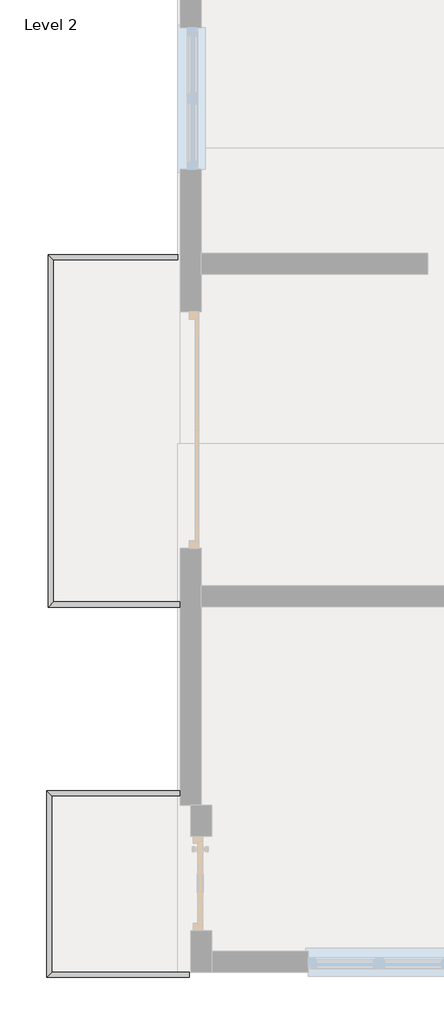
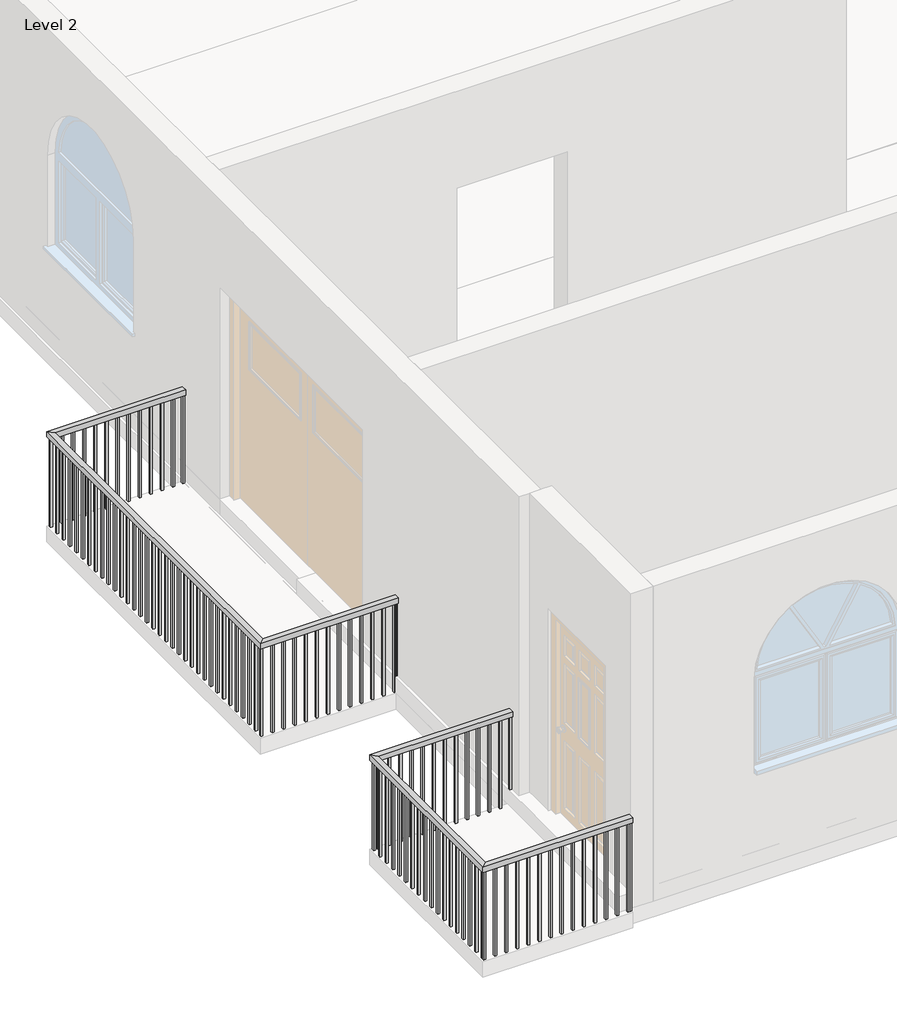
# One storey, part 3 of 7: 2 railings.
"""IFC4 building model written with IfcOpenShell, lengths in millimetres."""

from ifc_helpers import new_model, si_unit, frame, origin, place, context, project, spatial, polyline, outline, extrude, faceted_brep, element, save

model = new_model("IFC4")

# Units and contexts
model_context = context("Model", 3, world=origin())
ifc_project = project(units=[si_unit("LENGTHUNIT", "METRE", prefix="MILLI")], contexts=[model_context])

# Site, building, storey
site = spatial("IfcSite", under=ifc_project)
building = spatial("IfcBuilding", under=site)
storey = spatial("IfcBuildingStorey", under=building, Name="Level 2", Elevation=3048.0)

# Railings
placement = place(None, origin())
element("IfcRailing", 1, ObjectType="Handrail - Rectangular", at=placement, inside=storey, context=model_context, shape_type="SolidModel", body=[
    faceted_brep([(-6354.2109037, -3767.6037749, 3962.4), (-6354.2109037, -3767.6037749, 3911.6), (-6354.2109037, -3716.8037749, 3911.6), (-6354.2109037, -3716.8037749, 3962.4), (-7548.0109037, -3767.6037749, 3962.4), (-7548.0109037, -3767.6037749, 3911.6), (-7598.8109037, -3716.8037749, 3911.6), (-7598.8109037, -3716.8037749, 3962.4), (-7548.0109037, -7054.4894702, 3962.4), (-7548.0109037, -7054.4894702, 3911.6), (-7598.8109037, -7105.2894702, 3911.6), (-7598.8109037, -7105.2894702, 3962.4), (-6330.8013636, -7054.4894702, 3962.4), (-6330.8013636, -7105.2894702, 3962.4), (-6330.8013636, -7105.2894702, 3911.6), (-6330.8013636, -7054.4894702, 3911.6)], [[[0, 1, 2, 3]], [[1, 0, 4, 5]], [[2, 1, 5, 6]], [[3, 2, 6, 7]], [[0, 3, 7, 4]], [[5, 4, 8, 9]], [[6, 5, 9, 10]], [[7, 6, 10, 11]], [[4, 7, 11, 8]], [[12, 13, 14, 15]], [[9, 8, 12, 15]], [[10, 9, 15, 14]], [[11, 10, 14, 13]], [[8, 11, 13, 12]]]),
    extrude(outline(polyline([(-6363.7359037, -7089.4144702), (-6363.7359037, -7070.3644702), (-6344.6859037, -7070.3644702), (-6344.6859037, -7089.4144702), (-6363.7359037, -7089.4144702)])), frame((0.0, 0.0, 3048.0), z_axis=(0.0, 0.0, 1.0), x_axis=(1.0, 0.0, 0.0)), (0.0, 0.0, 1.0), 863.6),
    extrude(outline(polyline([(-6465.3359037, -7089.4144702), (-6465.3359037, -7070.3644702), (-6446.2859037, -7070.3644702), (-6446.2859037, -7089.4144702), (-6465.3359037, -7089.4144702)])), frame((0.0, 0.0, 3048.0), z_axis=(0.0, 0.0, 1.0), x_axis=(1.0, 0.0, 0.0)), (0.0, 0.0, 1.0), 863.6),
    extrude(outline(polyline([(-6566.9359037, -7089.4144702), (-6566.9359037, -7070.3644702), (-6547.8859037, -7070.3644702), (-6547.8859037, -7089.4144702), (-6566.9359037, -7089.4144702)])), frame((0.0, 0.0, 3048.0), z_axis=(0.0, 0.0, 1.0), x_axis=(1.0, 0.0, 0.0)), (0.0, 0.0, 1.0), 863.6),
    extrude(outline(polyline([(-6668.5359037, -7089.4144702), (-6668.5359037, -7070.3644702), (-6649.4859037, -7070.3644702), (-6649.4859037, -7089.4144702), (-6668.5359037, -7089.4144702)])), frame((0.0, 0.0, 3048.0), z_axis=(0.0, 0.0, 1.0), x_axis=(1.0, 0.0, 0.0)), (0.0, 0.0, 1.0), 863.6),
    extrude(outline(polyline([(-6770.1359037, -7089.4144702), (-6770.1359037, -7070.3644702), (-6751.0859037, -7070.3644702), (-6751.0859037, -7089.4144702), (-6770.1359037, -7089.4144702)])), frame((0.0, 0.0, 3048.0), z_axis=(0.0, 0.0, 1.0), x_axis=(1.0, 0.0, 0.0)), (0.0, 0.0, 1.0), 863.6),
    extrude(outline(polyline([(-6871.7359037, -7089.4144702), (-6871.7359037, -7070.3644702), (-6852.6859037, -7070.3644702), (-6852.6859037, -7089.4144702), (-6871.7359037, -7089.4144702)])), frame((0.0, 0.0, 3048.0), z_axis=(0.0, 0.0, 1.0), x_axis=(1.0, 0.0, 0.0)), (0.0, 0.0, 1.0), 863.6),
    extrude(outline(polyline([(-6973.3359037, -7089.4144702), (-6973.3359037, -7070.3644702), (-6954.2859037, -7070.3644702), (-6954.2859037, -7089.4144702), (-6973.3359037, -7089.4144702)])), frame((0.0, 0.0, 3048.0), z_axis=(0.0, 0.0, 1.0), x_axis=(1.0, 0.0, 0.0)), (0.0, 0.0, 1.0), 863.6),
    extrude(outline(polyline([(-7074.9359037, -7089.4144702), (-7074.9359037, -7070.3644702), (-7055.8859037, -7070.3644702), (-7055.8859037, -7089.4144702), (-7074.9359037, -7089.4144702)])), frame((0.0, 0.0, 3048.0), z_axis=(0.0, 0.0, 1.0), x_axis=(1.0, 0.0, 0.0)), (0.0, 0.0, 1.0), 863.6),
    extrude(outline(polyline([(-7176.5359037, -7089.4144702), (-7176.5359037, -7070.3644702), (-7157.4859037, -7070.3644702), (-7157.4859037, -7089.4144702), (-7176.5359037, -7089.4144702)])), frame((0.0, 0.0, 3048.0), z_axis=(0.0, 0.0, 1.0), x_axis=(1.0, 0.0, 0.0)), (0.0, 0.0, 1.0), 863.6),
    extrude(outline(polyline([(-7278.1359037, -7089.4144702), (-7278.1359037, -7070.3644702), (-7259.0859037, -7070.3644702), (-7259.0859037, -7089.4144702), (-7278.1359037, -7089.4144702)])), frame((0.0, 0.0, 3048.0), z_axis=(0.0, 0.0, 1.0), x_axis=(1.0, 0.0, 0.0)), (0.0, 0.0, 1.0), 863.6),
    extrude(outline(polyline([(-7379.7359037, -7089.4144702), (-7379.7359037, -7070.3644702), (-7360.6859037, -7070.3644702), (-7360.6859037, -7089.4144702), (-7379.7359037, -7089.4144702)])), frame((0.0, 0.0, 3048.0), z_axis=(0.0, 0.0, 1.0), x_axis=(1.0, 0.0, 0.0)), (0.0, 0.0, 1.0), 863.6),
    extrude(outline(polyline([(-7481.3359037, -7089.4144702), (-7481.3359037, -7070.3644702), (-7462.2859037, -7070.3644702), (-7462.2859037, -7089.4144702), (-7481.3359037, -7089.4144702)])), frame((0.0, 0.0, 3048.0), z_axis=(0.0, 0.0, 1.0), x_axis=(1.0, 0.0, 0.0)), (0.0, 0.0, 1.0), 863.6),
    extrude(outline(polyline([(-7582.9359037, -6983.8787749), (-7563.8859037, -6983.8787749), (-7563.8859037, -7002.9287749), (-7582.9359037, -7002.9287749), (-7582.9359037, -6983.8787749)])), frame((0.0, 0.0, 3048.0), z_axis=(0.0, 0.0, 1.0), x_axis=(1.0, 0.0, 0.0)), (0.0, 0.0, 1.0), 863.6),
    extrude(outline(polyline([(-7582.9359037, -6882.2787749), (-7563.8859037, -6882.2787749), (-7563.8859037, -6901.3287749), (-7582.9359037, -6901.3287749), (-7582.9359037, -6882.2787749)])), frame((0.0, 0.0, 3048.0), z_axis=(0.0, 0.0, 1.0), x_axis=(1.0, 0.0, 0.0)), (0.0, 0.0, 1.0), 863.6),
    extrude(outline(polyline([(-7582.9359037, -6780.6787749), (-7563.8859037, -6780.6787749), (-7563.8859037, -6799.7287749), (-7582.9359037, -6799.7287749), (-7582.9359037, -6780.6787749)])), frame((0.0, 0.0, 3048.0), z_axis=(0.0, 0.0, 1.0), x_axis=(1.0, 0.0, 0.0)), (0.0, 0.0, 1.0), 863.6),
    extrude(outline(polyline([(-7582.9359037, -6679.0787749), (-7563.8859037, -6679.0787749), (-7563.8859037, -6698.1287749), (-7582.9359037, -6698.1287749), (-7582.9359037, -6679.0787749)])), frame((0.0, 0.0, 3048.0), z_axis=(0.0, 0.0, 1.0), x_axis=(1.0, 0.0, 0.0)), (0.0, 0.0, 1.0), 863.6),
    extrude(outline(polyline([(-7582.9359037, -6577.4787749), (-7563.8859037, -6577.4787749), (-7563.8859037, -6596.5287749), (-7582.9359037, -6596.5287749), (-7582.9359037, -6577.4787749)])), frame((0.0, 0.0, 3048.0), z_axis=(0.0, 0.0, 1.0), x_axis=(1.0, 0.0, 0.0)), (0.0, 0.0, 1.0), 863.6),
    extrude(outline(polyline([(-7582.9359037, -6475.8787749), (-7563.8859037, -6475.8787749), (-7563.8859037, -6494.9287749), (-7582.9359037, -6494.9287749), (-7582.9359037, -6475.8787749)])), frame((0.0, 0.0, 3048.0), z_axis=(0.0, 0.0, 1.0), x_axis=(1.0, 0.0, 0.0)), (0.0, 0.0, 1.0), 863.6),
    extrude(outline(polyline([(-7582.9359037, -6374.2787749), (-7563.8859037, -6374.2787749), (-7563.8859037, -6393.3287749), (-7582.9359037, -6393.3287749), (-7582.9359037, -6374.2787749)])), frame((0.0, 0.0, 3048.0), z_axis=(0.0, 0.0, 1.0), x_axis=(1.0, 0.0, 0.0)), (0.0, 0.0, 1.0), 863.6),
    extrude(outline(polyline([(-7582.9359037, -6272.6787749), (-7563.8859037, -6272.6787749), (-7563.8859037, -6291.7287749), (-7582.9359037, -6291.7287749), (-7582.9359037, -6272.6787749)])), frame((0.0, 0.0, 3048.0), z_axis=(0.0, 0.0, 1.0), x_axis=(1.0, 0.0, 0.0)), (0.0, 0.0, 1.0), 863.6),
    extrude(outline(polyline([(-7582.9359037, -6171.0787749), (-7563.8859037, -6171.0787749), (-7563.8859037, -6190.1287749), (-7582.9359037, -6190.1287749), (-7582.9359037, -6171.0787749)])), frame((0.0, 0.0, 3048.0), z_axis=(0.0, 0.0, 1.0), x_axis=(1.0, 0.0, 0.0)), (0.0, 0.0, 1.0), 863.6),
    extrude(outline(polyline([(-7582.9359037, -6069.4787749), (-7563.8859037, -6069.4787749), (-7563.8859037, -6088.5287749), (-7582.9359037, -6088.5287749), (-7582.9359037, -6069.4787749)])), frame((0.0, 0.0, 3048.0), z_axis=(0.0, 0.0, 1.0), x_axis=(1.0, 0.0, 0.0)), (0.0, 0.0, 1.0), 863.6),
    extrude(outline(polyline([(-7582.9359037, -5967.8787749), (-7563.8859037, -5967.8787749), (-7563.8859037, -5986.9287749), (-7582.9359037, -5986.9287749), (-7582.9359037, -5967.8787749)])), frame((0.0, 0.0, 3048.0), z_axis=(0.0, 0.0, 1.0), x_axis=(1.0, 0.0, 0.0)), (0.0, 0.0, 1.0), 863.6),
    extrude(outline(polyline([(-7582.9359037, -5866.2787749), (-7563.8859037, -5866.2787749), (-7563.8859037, -5885.3287749), (-7582.9359037, -5885.3287749), (-7582.9359037, -5866.2787749)])), frame((0.0, 0.0, 3048.0), z_axis=(0.0, 0.0, 1.0), x_axis=(1.0, 0.0, 0.0)), (0.0, 0.0, 1.0), 863.6),
    extrude(outline(polyline([(-7582.9359037, -5764.6787749), (-7563.8859037, -5764.6787749), (-7563.8859037, -5783.7287749), (-7582.9359037, -5783.7287749), (-7582.9359037, -5764.6787749)])), frame((0.0, 0.0, 3048.0), z_axis=(0.0, 0.0, 1.0), x_axis=(1.0, 0.0, 0.0)), (0.0, 0.0, 1.0), 863.6),
    extrude(outline(polyline([(-7582.9359037, -5663.0787749), (-7563.8859037, -5663.0787749), (-7563.8859037, -5682.1287749), (-7582.9359037, -5682.1287749), (-7582.9359037, -5663.0787749)])), frame((0.0, 0.0, 3048.0), z_axis=(0.0, 0.0, 1.0), x_axis=(1.0, 0.0, 0.0)), (0.0, 0.0, 1.0), 863.6),
    extrude(outline(polyline([(-7582.9359037, -5561.4787749), (-7563.8859037, -5561.4787749), (-7563.8859037, -5580.5287749), (-7582.9359037, -5580.5287749), (-7582.9359037, -5561.4787749)])), frame((0.0, 0.0, 3048.0), z_axis=(0.0, 0.0, 1.0), x_axis=(1.0, 0.0, 0.0)), (0.0, 0.0, 1.0), 863.6),
    extrude(outline(polyline([(-7582.9359037, -5459.8787749), (-7563.8859037, -5459.8787749), (-7563.8859037, -5478.9287749), (-7582.9359037, -5478.9287749), (-7582.9359037, -5459.8787749)])), frame((0.0, 0.0, 3048.0), z_axis=(0.0, 0.0, 1.0), x_axis=(1.0, 0.0, 0.0)), (0.0, 0.0, 1.0), 863.6),
    extrude(outline(polyline([(-7582.9359037, -5358.2787749), (-7563.8859037, -5358.2787749), (-7563.8859037, -5377.3287749), (-7582.9359037, -5377.3287749), (-7582.9359037, -5358.2787749)])), frame((0.0, 0.0, 3048.0), z_axis=(0.0, 0.0, 1.0), x_axis=(1.0, 0.0, 0.0)), (0.0, 0.0, 1.0), 863.6),
    extrude(outline(polyline([(-7582.9359037, -5256.6787749), (-7563.8859037, -5256.6787749), (-7563.8859037, -5275.7287749), (-7582.9359037, -5275.7287749), (-7582.9359037, -5256.6787749)])), frame((0.0, 0.0, 3048.0), z_axis=(0.0, 0.0, 1.0), x_axis=(1.0, 0.0, 0.0)), (0.0, 0.0, 1.0), 863.6),
    extrude(outline(polyline([(-7582.9359037, -5155.0787749), (-7563.8859037, -5155.0787749), (-7563.8859037, -5174.1287749), (-7582.9359037, -5174.1287749), (-7582.9359037, -5155.0787749)])), frame((0.0, 0.0, 3048.0), z_axis=(0.0, 0.0, 1.0), x_axis=(1.0, 0.0, 0.0)), (0.0, 0.0, 1.0), 863.6),
    extrude(outline(polyline([(-7582.9359037, -5053.4787749), (-7563.8859037, -5053.4787749), (-7563.8859037, -5072.5287749), (-7582.9359037, -5072.5287749), (-7582.9359037, -5053.4787749)])), frame((0.0, 0.0, 3048.0), z_axis=(0.0, 0.0, 1.0), x_axis=(1.0, 0.0, 0.0)), (0.0, 0.0, 1.0), 863.6),
    extrude(outline(polyline([(-7582.9359037, -4951.8787749), (-7563.8859037, -4951.8787749), (-7563.8859037, -4970.9287749), (-7582.9359037, -4970.9287749), (-7582.9359037, -4951.8787749)])), frame((0.0, 0.0, 3048.0), z_axis=(0.0, 0.0, 1.0), x_axis=(1.0, 0.0, 0.0)), (0.0, 0.0, 1.0), 863.6),
    extrude(outline(polyline([(-7582.9359037, -4850.2787749), (-7563.8859037, -4850.2787749), (-7563.8859037, -4869.3287749), (-7582.9359037, -4869.3287749), (-7582.9359037, -4850.2787749)])), frame((0.0, 0.0, 3048.0), z_axis=(0.0, 0.0, 1.0), x_axis=(1.0, 0.0, 0.0)), (0.0, 0.0, 1.0), 863.6),
    extrude(outline(polyline([(-7582.9359037, -4748.6787749), (-7563.8859037, -4748.6787749), (-7563.8859037, -4767.7287749), (-7582.9359037, -4767.7287749), (-7582.9359037, -4748.6787749)])), frame((0.0, 0.0, 3048.0), z_axis=(0.0, 0.0, 1.0), x_axis=(1.0, 0.0, 0.0)), (0.0, 0.0, 1.0), 863.6),
    extrude(outline(polyline([(-7582.9359037, -4647.0787749), (-7563.8859037, -4647.0787749), (-7563.8859037, -4666.1287749), (-7582.9359037, -4666.1287749), (-7582.9359037, -4647.0787749)])), frame((0.0, 0.0, 3048.0), z_axis=(0.0, 0.0, 1.0), x_axis=(1.0, 0.0, 0.0)), (0.0, 0.0, 1.0), 863.6),
    extrude(outline(polyline([(-7582.9359037, -4545.4787749), (-7563.8859037, -4545.4787749), (-7563.8859037, -4564.5287749), (-7582.9359037, -4564.5287749), (-7582.9359037, -4545.4787749)])), frame((0.0, 0.0, 3048.0), z_axis=(0.0, 0.0, 1.0), x_axis=(1.0, 0.0, 0.0)), (0.0, 0.0, 1.0), 863.6),
    extrude(outline(polyline([(-7582.9359037, -4443.8787749), (-7563.8859037, -4443.8787749), (-7563.8859037, -4462.9287749), (-7582.9359037, -4462.9287749), (-7582.9359037, -4443.8787749)])), frame((0.0, 0.0, 3048.0), z_axis=(0.0, 0.0, 1.0), x_axis=(1.0, 0.0, 0.0)), (0.0, 0.0, 1.0), 863.6),
    extrude(outline(polyline([(-7582.9359037, -4342.2787749), (-7563.8859037, -4342.2787749), (-7563.8859037, -4361.3287749), (-7582.9359037, -4361.3287749), (-7582.9359037, -4342.2787749)])), frame((0.0, 0.0, 3048.0), z_axis=(0.0, 0.0, 1.0), x_axis=(1.0, 0.0, 0.0)), (0.0, 0.0, 1.0), 863.6),
    extrude(outline(polyline([(-7582.9359037, -4240.6787749), (-7563.8859037, -4240.6787749), (-7563.8859037, -4259.7287749), (-7582.9359037, -4259.7287749), (-7582.9359037, -4240.6787749)])), frame((0.0, 0.0, 3048.0), z_axis=(0.0, 0.0, 1.0), x_axis=(1.0, 0.0, 0.0)), (0.0, 0.0, 1.0), 863.6),
    extrude(outline(polyline([(-7582.9359037, -4139.0787749), (-7563.8859037, -4139.0787749), (-7563.8859037, -4158.1287749), (-7582.9359037, -4158.1287749), (-7582.9359037, -4139.0787749)])), frame((0.0, 0.0, 3048.0), z_axis=(0.0, 0.0, 1.0), x_axis=(1.0, 0.0, 0.0)), (0.0, 0.0, 1.0), 863.6),
    extrude(outline(polyline([(-7582.9359037, -4037.4787749), (-7563.8859037, -4037.4787749), (-7563.8859037, -4056.5287749), (-7582.9359037, -4056.5287749), (-7582.9359037, -4037.4787749)])), frame((0.0, 0.0, 3048.0), z_axis=(0.0, 0.0, 1.0), x_axis=(1.0, 0.0, 0.0)), (0.0, 0.0, 1.0), 863.6),
    extrude(outline(polyline([(-7582.9359037, -3935.8787749), (-7563.8859037, -3935.8787749), (-7563.8859037, -3954.9287749), (-7582.9359037, -3954.9287749), (-7582.9359037, -3935.8787749)])), frame((0.0, 0.0, 3048.0), z_axis=(0.0, 0.0, 1.0), x_axis=(1.0, 0.0, 0.0)), (0.0, 0.0, 1.0), 863.6),
    extrude(outline(polyline([(-7582.9359037, -3834.2787749), (-7563.8859037, -3834.2787749), (-7563.8859037, -3853.3287749), (-7582.9359037, -3853.3287749), (-7582.9359037, -3834.2787749)])), frame((0.0, 0.0, 3048.0), z_axis=(0.0, 0.0, 1.0), x_axis=(1.0, 0.0, 0.0)), (0.0, 0.0, 1.0), 863.6),
    extrude(outline(polyline([(-7462.2859037, -3732.6787749), (-7462.2859037, -3751.7287749), (-7481.3359037, -3751.7287749), (-7481.3359037, -3732.6787749), (-7462.2859037, -3732.6787749)])), frame((0.0, 0.0, 3048.0), z_axis=(0.0, 0.0, 1.0), x_axis=(1.0, 0.0, 0.0)), (0.0, 0.0, 1.0), 863.6),
    extrude(outline(polyline([(-7360.6859037, -3732.6787749), (-7360.6859037, -3751.7287749), (-7379.7359037, -3751.7287749), (-7379.7359037, -3732.6787749), (-7360.6859037, -3732.6787749)])), frame((0.0, 0.0, 3048.0), z_axis=(0.0, 0.0, 1.0), x_axis=(1.0, 0.0, 0.0)), (0.0, 0.0, 1.0), 863.6),
    extrude(outline(polyline([(-7259.0859037, -3732.6787749), (-7259.0859037, -3751.7287749), (-7278.1359037, -3751.7287749), (-7278.1359037, -3732.6787749), (-7259.0859037, -3732.6787749)])), frame((0.0, 0.0, 3048.0), z_axis=(0.0, 0.0, 1.0), x_axis=(1.0, 0.0, 0.0)), (0.0, 0.0, 1.0), 863.6),
    extrude(outline(polyline([(-7157.4859037, -3732.6787749), (-7157.4859037, -3751.7287749), (-7176.5359037, -3751.7287749), (-7176.5359037, -3732.6787749), (-7157.4859037, -3732.6787749)])), frame((0.0, 0.0, 3048.0), z_axis=(0.0, 0.0, 1.0), x_axis=(1.0, 0.0, 0.0)), (0.0, 0.0, 1.0), 863.6),
    extrude(outline(polyline([(-7055.8859037, -3732.6787749), (-7055.8859037, -3751.7287749), (-7074.9359037, -3751.7287749), (-7074.9359037, -3732.6787749), (-7055.8859037, -3732.6787749)])), frame((0.0, 0.0, 3048.0), z_axis=(0.0, 0.0, 1.0), x_axis=(1.0, 0.0, 0.0)), (0.0, 0.0, 1.0), 863.6),
    extrude(outline(polyline([(-6954.2859037, -3732.6787749), (-6954.2859037, -3751.7287749), (-6973.3359037, -3751.7287749), (-6973.3359037, -3732.6787749), (-6954.2859037, -3732.6787749)])), frame((0.0, 0.0, 3048.0), z_axis=(0.0, 0.0, 1.0), x_axis=(1.0, 0.0, 0.0)), (0.0, 0.0, 1.0), 863.6),
    extrude(outline(polyline([(-6852.6859037, -3732.6787749), (-6852.6859037, -3751.7287749), (-6871.7359037, -3751.7287749), (-6871.7359037, -3732.6787749), (-6852.6859037, -3732.6787749)])), frame((0.0, 0.0, 3048.0), z_axis=(0.0, 0.0, 1.0), x_axis=(1.0, 0.0, 0.0)), (0.0, 0.0, 1.0), 863.6),
    extrude(outline(polyline([(-6751.0859037, -3732.6787749), (-6751.0859037, -3751.7287749), (-6770.1359037, -3751.7287749), (-6770.1359037, -3732.6787749), (-6751.0859037, -3732.6787749)])), frame((0.0, 0.0, 3048.0), z_axis=(0.0, 0.0, 1.0), x_axis=(1.0, 0.0, 0.0)), (0.0, 0.0, 1.0), 863.6),
    extrude(outline(polyline([(-6649.4859037, -3732.6787749), (-6649.4859037, -3751.7287749), (-6668.5359037, -3751.7287749), (-6668.5359037, -3732.6787749), (-6649.4859037, -3732.6787749)])), frame((0.0, 0.0, 3048.0), z_axis=(0.0, 0.0, 1.0), x_axis=(1.0, 0.0, 0.0)), (0.0, 0.0, 1.0), 863.6),
    extrude(outline(polyline([(-6547.8859037, -3732.6787749), (-6547.8859037, -3751.7287749), (-6566.9359037, -3751.7287749), (-6566.9359037, -3732.6787749), (-6547.8859037, -3732.6787749)])), frame((0.0, 0.0, 3048.0), z_axis=(0.0, 0.0, 1.0), x_axis=(1.0, 0.0, 0.0)), (0.0, 0.0, 1.0), 863.6),
    extrude(outline(polyline([(-6446.2859037, -3732.6787749), (-6446.2859037, -3751.7287749), (-6465.3359037, -3751.7287749), (-6465.3359037, -3732.6787749), (-6446.2859037, -3732.6787749)])), frame((0.0, 0.0, 3048.0), z_axis=(0.0, 0.0, 1.0), x_axis=(1.0, 0.0, 0.0)), (0.0, 0.0, 1.0), 863.6),
    extrude(outline(polyline([(-7582.9359037, -7070.3644702), (-7563.8859037, -7070.3644702), (-7563.8859037, -7089.4144702), (-7582.9359037, -7089.4144702), (-7582.9359037, -7070.3644702)])), frame((0.0, 0.0, 3048.0), z_axis=(0.0, 0.0, 1.0), x_axis=(1.0, 0.0, 0.0)), (0.0, 0.0, 1.0), 863.6),
    extrude(outline(polyline([(-7563.8859037, -3732.6787749), (-7563.8859037, -3751.7287749), (-7582.9359037, -3751.7287749), (-7582.9359037, -3732.6787749), (-7563.8859037, -3732.6787749)])), frame((0.0, 0.0, 3048.0), z_axis=(0.0, 0.0, 1.0), x_axis=(1.0, 0.0, 0.0)), (0.0, 0.0, 1.0), 863.6),
    extrude(outline(polyline([(-6349.8513636, -7089.4144702), (-6349.8513636, -7070.3644702), (-6330.8013636, -7070.3644702), (-6330.8013636, -7089.4144702), (-6349.8513636, -7089.4144702)])), frame((0.0, 0.0, 3048.0), z_axis=(0.0, 0.0, 1.0), x_axis=(1.0, 0.0, 0.0)), (0.0, 0.0, 1.0), 863.6),
    extrude(outline(polyline([(-6354.2109037, -3732.6787749), (-6354.2109037, -3751.7287749), (-6373.2609037, -3751.7287749), (-6373.2609037, -3732.6787749), (-6354.2109037, -3732.6787749)])), frame((0.0, 0.0, 3048.0), z_axis=(0.0, 0.0, 1.0), x_axis=(1.0, 0.0, 0.0)), (0.0, 0.0, 1.0), 863.6),
])
element("IfcRailing", 2, ObjectType="Handrail - Rectangular", at=placement, inside=storey, context=model_context, shape_type="SolidModel", body=[
    faceted_brep([(-6330.8013636, -8918.8845215, 3962.4), (-6330.8013636, -8918.8845215, 3911.6), (-6330.8013636, -8868.0845215, 3911.6), (-6330.8013636, -8868.0845215, 3962.4), (-7563.8859037, -8918.8845215, 3962.4), (-7563.8859037, -8918.8845215, 3911.6), (-7614.6859037, -8868.0845215, 3911.6), (-7614.6859037, -8868.0845215, 3962.4), (-7563.8859037, -10612.9037749, 3962.4), (-7563.8859037, -10612.9037749, 3911.6), (-7614.6859037, -10663.7037749, 3911.6), (-7614.6859037, -10663.7037749, 3962.4), (-6243.0859037, -10612.9037749, 3962.4), (-6243.0859037, -10663.7037749, 3962.4), (-6243.0859037, -10663.7037749, 3911.6), (-6243.0859037, -10612.9037749, 3911.6)], [[[0, 1, 2, 3]], [[1, 0, 4, 5]], [[2, 1, 5, 6]], [[3, 2, 6, 7]], [[0, 3, 7, 4]], [[5, 4, 8, 9]], [[6, 5, 9, 10]], [[7, 6, 10, 11]], [[4, 7, 11, 8]], [[12, 13, 14, 15]], [[9, 8, 12, 15]], [[10, 9, 15, 14]], [[11, 10, 14, 13]], [[8, 11, 13, 12]]]),
    extrude(outline(polyline([(-6278.0109037, -10647.8287749), (-6278.0109037, -10628.7787749), (-6258.9609037, -10628.7787749), (-6258.9609037, -10647.8287749), (-6278.0109037, -10647.8287749)])), frame((0.0, 0.0, 3048.0), z_axis=(0.0, 0.0, 1.0), x_axis=(1.0, 0.0, 0.0)), (0.0, 0.0, 1.0), 863.6),
    extrude(outline(polyline([(-6379.6109037, -10647.8287749), (-6379.6109037, -10628.7787749), (-6360.5609037, -10628.7787749), (-6360.5609037, -10647.8287749), (-6379.6109037, -10647.8287749)])), frame((0.0, 0.0, 3048.0), z_axis=(0.0, 0.0, 1.0), x_axis=(1.0, 0.0, 0.0)), (0.0, 0.0, 1.0), 863.6),
    extrude(outline(polyline([(-6481.2109037, -10647.8287749), (-6481.2109037, -10628.7787749), (-6462.1609037, -10628.7787749), (-6462.1609037, -10647.8287749), (-6481.2109037, -10647.8287749)])), frame((0.0, 0.0, 3048.0), z_axis=(0.0, 0.0, 1.0), x_axis=(1.0, 0.0, 0.0)), (0.0, 0.0, 1.0), 863.6),
    extrude(outline(polyline([(-6582.8109037, -10647.8287749), (-6582.8109037, -10628.7787749), (-6563.7609037, -10628.7787749), (-6563.7609037, -10647.8287749), (-6582.8109037, -10647.8287749)])), frame((0.0, 0.0, 3048.0), z_axis=(0.0, 0.0, 1.0), x_axis=(1.0, 0.0, 0.0)), (0.0, 0.0, 1.0), 863.6),
    extrude(outline(polyline([(-6684.4109037, -10647.8287749), (-6684.4109037, -10628.7787749), (-6665.3609037, -10628.7787749), (-6665.3609037, -10647.8287749), (-6684.4109037, -10647.8287749)])), frame((0.0, 0.0, 3048.0), z_axis=(0.0, 0.0, 1.0), x_axis=(1.0, 0.0, 0.0)), (0.0, 0.0, 1.0), 863.6),
    extrude(outline(polyline([(-6786.0109037, -10647.8287749), (-6786.0109037, -10628.7787749), (-6766.9609037, -10628.7787749), (-6766.9609037, -10647.8287749), (-6786.0109037, -10647.8287749)])), frame((0.0, 0.0, 3048.0), z_axis=(0.0, 0.0, 1.0), x_axis=(1.0, 0.0, 0.0)), (0.0, 0.0, 1.0), 863.6),
    extrude(outline(polyline([(-6887.6109037, -10647.8287749), (-6887.6109037, -10628.7787749), (-6868.5609037, -10628.7787749), (-6868.5609037, -10647.8287749), (-6887.6109037, -10647.8287749)])), frame((0.0, 0.0, 3048.0), z_axis=(0.0, 0.0, 1.0), x_axis=(1.0, 0.0, 0.0)), (0.0, 0.0, 1.0), 863.6),
    extrude(outline(polyline([(-6989.2109037, -10647.8287749), (-6989.2109037, -10628.7787749), (-6970.1609037, -10628.7787749), (-6970.1609037, -10647.8287749), (-6989.2109037, -10647.8287749)])), frame((0.0, 0.0, 3048.0), z_axis=(0.0, 0.0, 1.0), x_axis=(1.0, 0.0, 0.0)), (0.0, 0.0, 1.0), 863.6),
    extrude(outline(polyline([(-7090.8109037, -10647.8287749), (-7090.8109037, -10628.7787749), (-7071.7609037, -10628.7787749), (-7071.7609037, -10647.8287749), (-7090.8109037, -10647.8287749)])), frame((0.0, 0.0, 3048.0), z_axis=(0.0, 0.0, 1.0), x_axis=(1.0, 0.0, 0.0)), (0.0, 0.0, 1.0), 863.6),
    extrude(outline(polyline([(-7192.4109037, -10647.8287749), (-7192.4109037, -10628.7787749), (-7173.3609037, -10628.7787749), (-7173.3609037, -10647.8287749), (-7192.4109037, -10647.8287749)])), frame((0.0, 0.0, 3048.0), z_axis=(0.0, 0.0, 1.0), x_axis=(1.0, 0.0, 0.0)), (0.0, 0.0, 1.0), 863.6),
    extrude(outline(polyline([(-7294.0109037, -10647.8287749), (-7294.0109037, -10628.7787749), (-7274.9609037, -10628.7787749), (-7274.9609037, -10647.8287749), (-7294.0109037, -10647.8287749)])), frame((0.0, 0.0, 3048.0), z_axis=(0.0, 0.0, 1.0), x_axis=(1.0, 0.0, 0.0)), (0.0, 0.0, 1.0), 863.6),
    extrude(outline(polyline([(-7395.6109037, -10647.8287749), (-7395.6109037, -10628.7787749), (-7376.5609037, -10628.7787749), (-7376.5609037, -10647.8287749), (-7395.6109037, -10647.8287749)])), frame((0.0, 0.0, 3048.0), z_axis=(0.0, 0.0, 1.0), x_axis=(1.0, 0.0, 0.0)), (0.0, 0.0, 1.0), 863.6),
    extrude(outline(polyline([(-7497.2109037, -10647.8287749), (-7497.2109037, -10628.7787749), (-7478.1609037, -10628.7787749), (-7478.1609037, -10647.8287749), (-7497.2109037, -10647.8287749)])), frame((0.0, 0.0, 3048.0), z_axis=(0.0, 0.0, 1.0), x_axis=(1.0, 0.0, 0.0)), (0.0, 0.0, 1.0), 863.6),
    extrude(outline(polyline([(-7598.8109037, -10611.1595215), (-7579.7609037, -10611.1595215), (-7579.7609037, -10630.2095215), (-7598.8109037, -10630.2095215), (-7598.8109037, -10611.1595215)])), frame((0.0, 0.0, 3048.0), z_axis=(0.0, 0.0, 1.0), x_axis=(1.0, 0.0, 0.0)), (0.0, 0.0, 1.0), 863.6),
    extrude(outline(polyline([(-7598.8109037, -10509.5595215), (-7579.7609037, -10509.5595215), (-7579.7609037, -10528.6095215), (-7598.8109037, -10528.6095215), (-7598.8109037, -10509.5595215)])), frame((0.0, 0.0, 3048.0), z_axis=(0.0, 0.0, 1.0), x_axis=(1.0, 0.0, 0.0)), (0.0, 0.0, 1.0), 863.6),
    extrude(outline(polyline([(-7598.8109037, -10407.9595215), (-7579.7609037, -10407.9595215), (-7579.7609037, -10427.0095215), (-7598.8109037, -10427.0095215), (-7598.8109037, -10407.9595215)])), frame((0.0, 0.0, 3048.0), z_axis=(0.0, 0.0, 1.0), x_axis=(1.0, 0.0, 0.0)), (0.0, 0.0, 1.0), 863.6),
    extrude(outline(polyline([(-7598.8109037, -10306.3595215), (-7579.7609037, -10306.3595215), (-7579.7609037, -10325.4095215), (-7598.8109037, -10325.4095215), (-7598.8109037, -10306.3595215)])), frame((0.0, 0.0, 3048.0), z_axis=(0.0, 0.0, 1.0), x_axis=(1.0, 0.0, 0.0)), (0.0, 0.0, 1.0), 863.6),
    extrude(outline(polyline([(-7598.8109037, -10204.7595215), (-7579.7609037, -10204.7595215), (-7579.7609037, -10223.8095215), (-7598.8109037, -10223.8095215), (-7598.8109037, -10204.7595215)])), frame((0.0, 0.0, 3048.0), z_axis=(0.0, 0.0, 1.0), x_axis=(1.0, 0.0, 0.0)), (0.0, 0.0, 1.0), 863.6),
    extrude(outline(polyline([(-7598.8109037, -10103.1595215), (-7579.7609037, -10103.1595215), (-7579.7609037, -10122.2095215), (-7598.8109037, -10122.2095215), (-7598.8109037, -10103.1595215)])), frame((0.0, 0.0, 3048.0), z_axis=(0.0, 0.0, 1.0), x_axis=(1.0, 0.0, 0.0)), (0.0, 0.0, 1.0), 863.6),
    extrude(outline(polyline([(-7598.8109037, -10001.5595215), (-7579.7609037, -10001.5595215), (-7579.7609037, -10020.6095215), (-7598.8109037, -10020.6095215), (-7598.8109037, -10001.5595215)])), frame((0.0, 0.0, 3048.0), z_axis=(0.0, 0.0, 1.0), x_axis=(1.0, 0.0, 0.0)), (0.0, 0.0, 1.0), 863.6),
    extrude(outline(polyline([(-7598.8109037, -9899.9595215), (-7579.7609037, -9899.9595215), (-7579.7609037, -9919.0095215), (-7598.8109037, -9919.0095215), (-7598.8109037, -9899.9595215)])), frame((0.0, 0.0, 3048.0), z_axis=(0.0, 0.0, 1.0), x_axis=(1.0, 0.0, 0.0)), (0.0, 0.0, 1.0), 863.6),
    extrude(outline(polyline([(-7598.8109037, -9798.3595215), (-7579.7609037, -9798.3595215), (-7579.7609037, -9817.4095215), (-7598.8109037, -9817.4095215), (-7598.8109037, -9798.3595215)])), frame((0.0, 0.0, 3048.0), z_axis=(0.0, 0.0, 1.0), x_axis=(1.0, 0.0, 0.0)), (0.0, 0.0, 1.0), 863.6),
    extrude(outline(polyline([(-7598.8109037, -9696.7595215), (-7579.7609037, -9696.7595215), (-7579.7609037, -9715.8095215), (-7598.8109037, -9715.8095215), (-7598.8109037, -9696.7595215)])), frame((0.0, 0.0, 3048.0), z_axis=(0.0, 0.0, 1.0), x_axis=(1.0, 0.0, 0.0)), (0.0, 0.0, 1.0), 863.6),
    extrude(outline(polyline([(-7598.8109037, -9595.1595215), (-7579.7609037, -9595.1595215), (-7579.7609037, -9614.2095215), (-7598.8109037, -9614.2095215), (-7598.8109037, -9595.1595215)])), frame((0.0, 0.0, 3048.0), z_axis=(0.0, 0.0, 1.0), x_axis=(1.0, 0.0, 0.0)), (0.0, 0.0, 1.0), 863.6),
    extrude(outline(polyline([(-7598.8109037, -9493.5595215), (-7579.7609037, -9493.5595215), (-7579.7609037, -9512.6095215), (-7598.8109037, -9512.6095215), (-7598.8109037, -9493.5595215)])), frame((0.0, 0.0, 3048.0), z_axis=(0.0, 0.0, 1.0), x_axis=(1.0, 0.0, 0.0)), (0.0, 0.0, 1.0), 863.6),
    extrude(outline(polyline([(-7598.8109037, -9391.9595215), (-7579.7609037, -9391.9595215), (-7579.7609037, -9411.0095215), (-7598.8109037, -9411.0095215), (-7598.8109037, -9391.9595215)])), frame((0.0, 0.0, 3048.0), z_axis=(0.0, 0.0, 1.0), x_axis=(1.0, 0.0, 0.0)), (0.0, 0.0, 1.0), 863.6),
    extrude(outline(polyline([(-7598.8109037, -9290.3595215), (-7579.7609037, -9290.3595215), (-7579.7609037, -9309.4095215), (-7598.8109037, -9309.4095215), (-7598.8109037, -9290.3595215)])), frame((0.0, 0.0, 3048.0), z_axis=(0.0, 0.0, 1.0), x_axis=(1.0, 0.0, 0.0)), (0.0, 0.0, 1.0), 863.6),
    extrude(outline(polyline([(-7598.8109037, -9188.7595215), (-7579.7609037, -9188.7595215), (-7579.7609037, -9207.8095215), (-7598.8109037, -9207.8095215), (-7598.8109037, -9188.7595215)])), frame((0.0, 0.0, 3048.0), z_axis=(0.0, 0.0, 1.0), x_axis=(1.0, 0.0, 0.0)), (0.0, 0.0, 1.0), 863.6),
    extrude(outline(polyline([(-7598.8109037, -9087.1595215), (-7579.7609037, -9087.1595215), (-7579.7609037, -9106.2095215), (-7598.8109037, -9106.2095215), (-7598.8109037, -9087.1595215)])), frame((0.0, 0.0, 3048.0), z_axis=(0.0, 0.0, 1.0), x_axis=(1.0, 0.0, 0.0)), (0.0, 0.0, 1.0), 863.6),
    extrude(outline(polyline([(-7598.8109037, -8985.5595215), (-7579.7609037, -8985.5595215), (-7579.7609037, -9004.6095215), (-7598.8109037, -9004.6095215), (-7598.8109037, -8985.5595215)])), frame((0.0, 0.0, 3048.0), z_axis=(0.0, 0.0, 1.0), x_axis=(1.0, 0.0, 0.0)), (0.0, 0.0, 1.0), 863.6),
    extrude(outline(polyline([(-7540.4763636, -8883.9595215), (-7540.4763636, -8903.0095215), (-7559.5263636, -8903.0095215), (-7559.5263636, -8883.9595215), (-7540.4763636, -8883.9595215)])), frame((0.0, 0.0, 3048.0), z_axis=(0.0, 0.0, 1.0), x_axis=(1.0, 0.0, 0.0)), (0.0, 0.0, 1.0), 863.6),
    extrude(outline(polyline([(-7438.8763636, -8883.9595215), (-7438.8763636, -8903.0095215), (-7457.9263636, -8903.0095215), (-7457.9263636, -8883.9595215), (-7438.8763636, -8883.9595215)])), frame((0.0, 0.0, 3048.0), z_axis=(0.0, 0.0, 1.0), x_axis=(1.0, 0.0, 0.0)), (0.0, 0.0, 1.0), 863.6),
    extrude(outline(polyline([(-7337.2763636, -8883.9595215), (-7337.2763636, -8903.0095215), (-7356.3263636, -8903.0095215), (-7356.3263636, -8883.9595215), (-7337.2763636, -8883.9595215)])), frame((0.0, 0.0, 3048.0), z_axis=(0.0, 0.0, 1.0), x_axis=(1.0, 0.0, 0.0)), (0.0, 0.0, 1.0), 863.6),
    extrude(outline(polyline([(-7235.6763636, -8883.9595215), (-7235.6763636, -8903.0095215), (-7254.7263636, -8903.0095215), (-7254.7263636, -8883.9595215), (-7235.6763636, -8883.9595215)])), frame((0.0, 0.0, 3048.0), z_axis=(0.0, 0.0, 1.0), x_axis=(1.0, 0.0, 0.0)), (0.0, 0.0, 1.0), 863.6),
    extrude(outline(polyline([(-7134.0763636, -8883.9595215), (-7134.0763636, -8903.0095215), (-7153.1263636, -8903.0095215), (-7153.1263636, -8883.9595215), (-7134.0763636, -8883.9595215)])), frame((0.0, 0.0, 3048.0), z_axis=(0.0, 0.0, 1.0), x_axis=(1.0, 0.0, 0.0)), (0.0, 0.0, 1.0), 863.6),
    extrude(outline(polyline([(-7032.4763636, -8883.9595215), (-7032.4763636, -8903.0095215), (-7051.5263636, -8903.0095215), (-7051.5263636, -8883.9595215), (-7032.4763636, -8883.9595215)])), frame((0.0, 0.0, 3048.0), z_axis=(0.0, 0.0, 1.0), x_axis=(1.0, 0.0, 0.0)), (0.0, 0.0, 1.0), 863.6),
    extrude(outline(polyline([(-6930.8763636, -8883.9595215), (-6930.8763636, -8903.0095215), (-6949.9263636, -8903.0095215), (-6949.9263636, -8883.9595215), (-6930.8763636, -8883.9595215)])), frame((0.0, 0.0, 3048.0), z_axis=(0.0, 0.0, 1.0), x_axis=(1.0, 0.0, 0.0)), (0.0, 0.0, 1.0), 863.6),
    extrude(outline(polyline([(-6829.2763636, -8883.9595215), (-6829.2763636, -8903.0095215), (-6848.3263636, -8903.0095215), (-6848.3263636, -8883.9595215), (-6829.2763636, -8883.9595215)])), frame((0.0, 0.0, 3048.0), z_axis=(0.0, 0.0, 1.0), x_axis=(1.0, 0.0, 0.0)), (0.0, 0.0, 1.0), 863.6),
    extrude(outline(polyline([(-6727.6763636, -8883.9595215), (-6727.6763636, -8903.0095215), (-6746.7263636, -8903.0095215), (-6746.7263636, -8883.9595215), (-6727.6763636, -8883.9595215)])), frame((0.0, 0.0, 3048.0), z_axis=(0.0, 0.0, 1.0), x_axis=(1.0, 0.0, 0.0)), (0.0, 0.0, 1.0), 863.6),
    extrude(outline(polyline([(-6626.0763636, -8883.9595215), (-6626.0763636, -8903.0095215), (-6645.1263636, -8903.0095215), (-6645.1263636, -8883.9595215), (-6626.0763636, -8883.9595215)])), frame((0.0, 0.0, 3048.0), z_axis=(0.0, 0.0, 1.0), x_axis=(1.0, 0.0, 0.0)), (0.0, 0.0, 1.0), 863.6),
    extrude(outline(polyline([(-6524.4763636, -8883.9595215), (-6524.4763636, -8903.0095215), (-6543.5263636, -8903.0095215), (-6543.5263636, -8883.9595215), (-6524.4763636, -8883.9595215)])), frame((0.0, 0.0, 3048.0), z_axis=(0.0, 0.0, 1.0), x_axis=(1.0, 0.0, 0.0)), (0.0, 0.0, 1.0), 863.6),
    extrude(outline(polyline([(-6422.8763636, -8883.9595215), (-6422.8763636, -8903.0095215), (-6441.9263636, -8903.0095215), (-6441.9263636, -8883.9595215), (-6422.8763636, -8883.9595215)])), frame((0.0, 0.0, 3048.0), z_axis=(0.0, 0.0, 1.0), x_axis=(1.0, 0.0, 0.0)), (0.0, 0.0, 1.0), 863.6),
    extrude(outline(polyline([(-7598.8109037, -10628.7787749), (-7579.7609037, -10628.7787749), (-7579.7609037, -10647.8287749), (-7598.8109037, -10647.8287749), (-7598.8109037, -10628.7787749)])), frame((0.0, 0.0, 3048.0), z_axis=(0.0, 0.0, 1.0), x_axis=(1.0, 0.0, 0.0)), (0.0, 0.0, 1.0), 863.6),
    extrude(outline(polyline([(-7579.7609037, -8883.9595215), (-7579.7609037, -8903.0095215), (-7598.8109037, -8903.0095215), (-7598.8109037, -8883.9595215), (-7579.7609037, -8883.9595215)])), frame((0.0, 0.0, 3048.0), z_axis=(0.0, 0.0, 1.0), x_axis=(1.0, 0.0, 0.0)), (0.0, 0.0, 1.0), 863.6),
    extrude(outline(polyline([(-6262.1359037, -10647.8287749), (-6262.1359037, -10628.7787749), (-6243.0859037, -10628.7787749), (-6243.0859037, -10647.8287749), (-6262.1359037, -10647.8287749)])), frame((0.0, 0.0, 3048.0), z_axis=(0.0, 0.0, 1.0), x_axis=(1.0, 0.0, 0.0)), (0.0, 0.0, 1.0), 863.6),
    extrude(outline(polyline([(-6330.8013636, -8883.9595215), (-6330.8013636, -8903.0095215), (-6349.8513636, -8903.0095215), (-6349.8513636, -8883.9595215), (-6330.8013636, -8883.9595215)])), frame((0.0, 0.0, 3048.0), z_axis=(0.0, 0.0, 1.0), x_axis=(1.0, 0.0, 0.0)), (0.0, 0.0, 1.0), 863.6),
])

save(model, "model.ifc")

# Revit data of these elements
# Type "Handrail - Rectangular"
#   Assembly Code = "C2010400"
#   built-in parameter 1008612 = 0.0416667 (stored number, unit not read)
#   built-in parameter 1008611 = 0.0416667 (stored number, unit not read)
#   built-in parameter 1008609 = 0.333333 (stored number, unit not read)
#   built-in parameter 1008604 = 0.166667 (stored number, unit not read)
#   built-in parameter 1008603 = 0.166667 (stored number, unit not read)
#   Railing Height = 3' - 0"
#   built-in parameter 1008630 = 2
#   built-in parameter 1008610 = 2
#   built-in parameter 1008618 = Baluster - Square : 3/4"
# Elements 1, 2 (IfcRailing, "Handrail - Rectangular")
#   Phase Created = New Construction
